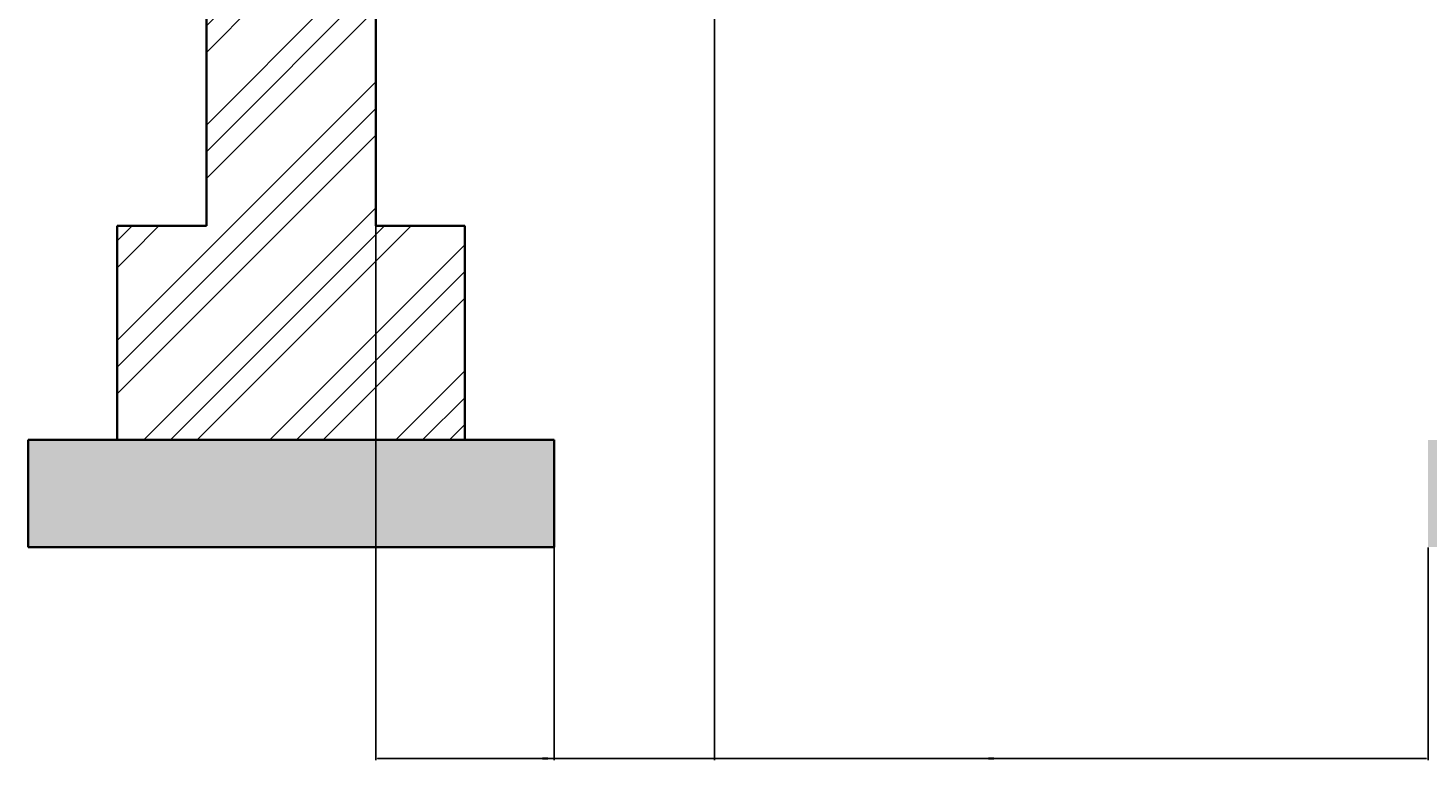
# Model space of a CAD drawing. Units: inches. Extents: x -128 to 854, y -395 to 398.
# Tile 13 of 61: x 122 to 279, y -382 to -300. Entities that reach past the tile are written whole.
import ezdxf

# ---------------------------------------------------------------- set-up
doc = ezdxf.new("R2010")
doc.units = ezdxf.units.IN
doc.header["$MEASUREMENT"] = 0
for name, color, linetype, lineweight in [('A-ANNO-DIMS', 2, 'Continuous', 18), ('A-SECT-PATT', 8, 'Continuous', 13), ('S-FNDN', 2, 'Continuous', 35), ('S-FNDN-PATT', 8, 'Continuous', 13)]:
    doc.layers.add(name, color=color, linetype=linetype, lineweight=lineweight)
doc.styles.get("Standard").update_dxf_attribs({"font": 'arial.ttf'})
doc.dimstyles.get("Standard").update_dxf_attribs({"dimtxt": 0.18, "dimasz": 0.18, "dimexe": 0.18, "dimexo": 0.0625, "dimgap": 0.09, "dimtad": 0, "dimtih": 1, "dimtoh": 1, "dimdec": 1, "dimzin": 0, "dimdsep": 46, "dimlunit": 4, "dimtxsty": 'Standard', "dimcen": 0.09, "dimclrd": 1, "dimclre": 2, "dimclrt": 6, "dimadec": 0, "dimazin": 0, "dimtfac": 1, "dimtdec": 1, "dimtofl": 0, "dimtmove": 0, "dimatfit": 3, "dimfxl": 1, "dimtfill": 2, "dimtfillclr": 3, "dimtolj": 1, "dimtzin": 0, "dimarcsym": 0})

# ---------------------------------------------------------------- blocks, each defined once
blk = doc.blocks.new('*D124')
at = {"layer": 'A-ANNO-DIMS', "color": 2, "lineweight": -2, "transparency": 16777216}
for p, q in [((180.84, -358.08), (180.84, -381.9)), ((278.84, -358.08), (278.84, -381.9))]:
    blk.add_line(p, q, dxfattribs=at)
at = {"layer": 'A-ANNO-DIMS', "color": 1, "lineweight": -2, "transparency": 16777216}
for p, q in [((181.02, -381.72), (229.51, -381.72)), ((278.66, -381.72), (230.17, -381.72))]:
    blk.add_line(p, q, dxfattribs=at)
at = {"layer": 'A-ANNO-DIMS', "color": 1, "transparency": 16777216}
for points in [[(181.02, -381.69), (181.02, -381.75), (180.84, -381.72)], [(278.66, -381.69), (278.66, -381.75), (278.84, -381.72)]]:
    blk.add_solid(points, dxfattribs=at)
at = {"layer": 'Defpoints', "color": 0, "transparency": 16777216}
for p in [(180.84, -358.02), (278.84, -358.02), (278.84, -381.72)]:
    blk.add_point(p, dxfattribs=at)
at = {"layer": 'A-ANNO-DIMS', "color": 6, "transparency": 16777216, "insert": (229.84, -381.72), "char_height": 0.18, "attachment_point": 5, "bg_fill": 1, "box_fill_scale": 1.25, "bg_fill_color": 3, "bg_fill_transparency": 0}
blk.add_mtext('\\A1;8\'-2"', dxfattribs=at)
blk = doc.blocks.new('*D126')
at = {"layer": 'A-ANNO-DIMS', "color": 2, "lineweight": -2, "transparency": 16777216}
for p, q in [((160.84, -178.08), (160.84, -381.9)), ((198.84, -202.08), (198.84, -381.9))]:
    blk.add_line(p, q, dxfattribs=at)
at = {"layer": 'A-ANNO-DIMS', "color": 1, "lineweight": -2, "transparency": 16777216}
for p, q in [((161.02, -381.72), (179.51, -381.72)), ((198.66, -381.72), (180.17, -381.72))]:
    blk.add_line(p, q, dxfattribs=at)
at = {"layer": 'A-ANNO-DIMS', "color": 1, "transparency": 16777216}
for points in [[(161.02, -381.69), (161.02, -381.75), (160.84, -381.72)], [(198.66, -381.69), (198.66, -381.75), (198.84, -381.72)]]:
    blk.add_solid(points, dxfattribs=at)
at = {"layer": 'Defpoints', "color": 0, "transparency": 16777216}
for p in [(160.84, -178.02), (198.84, -202.02), (198.84, -381.72)]:
    blk.add_point(p, dxfattribs=at)
at = {"layer": 'A-ANNO-DIMS', "color": 6, "transparency": 16777216, "insert": (179.84, -381.72), "char_height": 0.18, "attachment_point": 5, "bg_fill": 1, "box_fill_scale": 1.25, "bg_fill_color": 3, "bg_fill_transparency": 0}
blk.add_mtext('\\A1;3\'-2"', dxfattribs=at)

msp = doc.modelspace()

# ---------------------------------------------------------------- hatches: boundary and pattern name
at = {"layer": 'A-SECT-PATT'}
h = msp.add_hatch(dxfattribs=at)
h.set_pattern_fill('GOST_GROUND', color=256)
h.set_pattern_definition([(45, (0, 0), (14.14214, -9e-16), [20]), (45, (3, 0), (14.14214, -9e-16), [20]), (45, (6, 0), (14.14214, -9e-16), [20])])
h.paths.add_polyline_path([(-27.16, -322.02), (-37.16, -322.02), (-37.16, -298.02), (-56.16, -298.02), (-56.16, -322.02), (-66.16, -322.02), (-66.16, -346.02), (-27.16, -346.02)])
h.paths.add_polyline_path([(170.84, -322.02), (160.84, -322.02), (160.84, -298.02), (155.84, -298.02), (141.84, -298.02), (141.84, -322.02), (131.84, -322.02), (131.84, -346.02), (170.84, -346.02)])
h.paths.add_polyline_path([(327.84, -322.02), (317.84, -322.02), (317.84, -298.02), (312.84, -298.02), (298.84, -298.02), (298.84, -322.02), (288.84, -322.02), (288.84, -346.02), (327.84, -346.02)])
h.paths.add_polyline_path([(-37.16, -274.02), (-56.16, -274.02), (-56.16, -298.02), (-37.16, -298.02)])
h.paths.add_polyline_path([(-37.16, -207.02), (-56.16, -207.02), (-56.16, -226.02), (-37.16, -226.02)])
h.paths.add_polyline_path([(160.84, -274.02), (141.84, -274.02), (141.84, -298.02), (155.84, -298.02), (160.84, -298.02)])
at = {"layer": 'S-FNDN-PATT'}
h = msp.add_hatch(dxfattribs=at)
h.set_pattern_fill('AR-CONC', color=256)
h.paths.add_polyline_path([(-17.16, -346.02), (-27.16, -346.02), (-66.16, -346.02), (-76.16, -346.02), (-76.16, -358.02), (-17.16, -358.02)])
h.paths.add_polyline_path([(180.84, -346.02), (170.84, -346.02), (131.84, -346.02), (121.84, -346.02), (121.84, -358.02), (180.84, -358.02)])
h.paths.add_polyline_path([(337.84, -346.02), (327.84, -346.02), (288.84, -346.02), (278.84, -346.02), (278.84, -358.02), (337.84, -358.02)])

# ---------------------------------------------------------------- linework, layer by layer
at = {"layer": 'S-FNDN'}
for p, q in [((141.84, -298.02), (141.84, -322.02)), ((160.84, -298.02), (160.84, -322.02)), ((141.84, -322.02), (131.84, -322.02)), ((131.84, -322.02), (131.84, -346.02)), ((160.84, -322.02), (170.84, -322.02)), ((170.84, -322.02), (170.84, -346.02)), ((131.84, -346.02), (121.84, -346.02)), ((121.84, -346.02), (121.84, -358.02)), ((131.84, -346.02), (170.84, -346.02)), ((170.84, -346.02), (180.84, -346.02)), ((180.84, -346.02), (180.84, -358.02)), ((121.84, -358.02), (180.84, -358.02))]:
    msp.add_line(p, q, dxfattribs=at)

# ---------------------------------------------------------------- dimensions: what is measured, and where the dimension line sits
at = {"layer": 'A-ANNO-DIMS'}
for base, p1, p2, picture, middle in [((198.84, -381.72), (160.84, -178.02), (198.84, -202.02), '*D126', (179.84, -381.72)), ((278.84, -381.72), (180.84, -358.02), (278.84, -358.02), '*D124', (229.84, -381.72))]:
    dim = msp.add_linear_dim(base=base, p1=p1, p2=p2, dimstyle='Standard', override={"dimdec": 1, "dimlfac": 1, "dimrnd": 0, "dimzin": 1, "dimdsep": 46, "dimlunit": 4, "dimfrac": 2}, dxfattribs=at)
    dim.commit()
    dim.dimension.update_dxf_attribs({"geometry": picture, "text_midpoint": middle})

doc.saveas('drawing.dxf')
